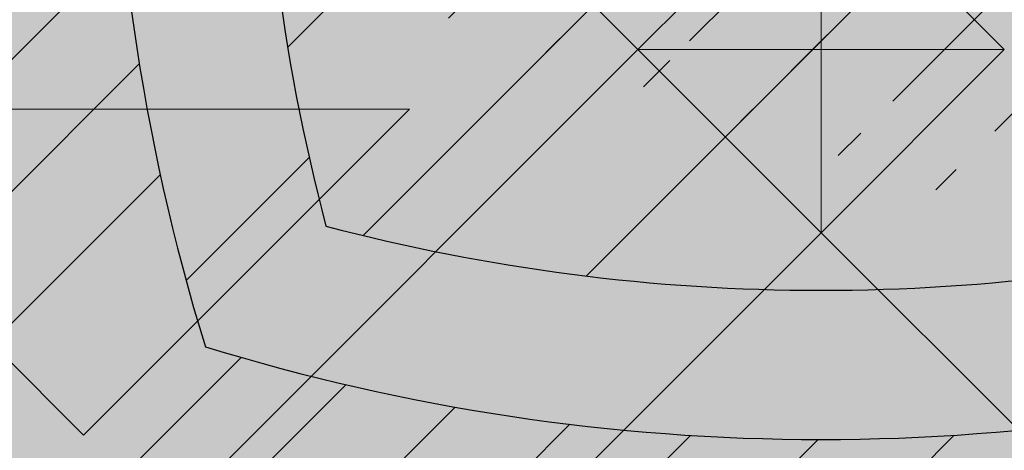
# Model space of a CAD drawing. Units: inches. Extents: x 844 to 2234, y 346 to 1084.
# Tile 10 of 93: x 1121.143 to 1123.249, y 690.263 to 691.183. Entities that reach past the tile are written whole.
import ezdxf

# ---------------------------------------------------------------- set-up
doc = ezdxf.new("R2010")
doc.units = ezdxf.units.IN
doc.header["$MEASUREMENT"] = 0
for name, color, linetype, lineweight in [('A-ANNO-DIMS', 2, 'Continuous', 18), ('furniture', 8, 'Continuous', 18), ('RA-AP-01$0$INT', 35, 'Continuous', 5)]:
    doc.layers.add(name, color=color, linetype=linetype, lineweight=lineweight)
doc.layers.add('RA-AP-01$0$FURN', color=3, linetype='Continuous')
doc.layers.add('RA-AP-01$0$WOOD', color=64, linetype='Continuous')
doc.styles.get("Standard").update_dxf_attribs({"font": 'arial.ttf'})
doc.dimstyles.get("Standard").update_dxf_attribs({"dimtxt": 6, "dimasz": 3, "dimexe": 0.18, "dimexo": 0.0625, "dimgap": 0.09, "dimtad": 0, "dimtih": 1, "dimtoh": 1, "dimdec": 1, "dimzin": 0, "dimdsep": 46, "dimlunit": 3, "dimtxsty": 'Standard', "dimblk": 'ARCHTICK', "dimcen": 0.09, "dimadec": 0, "dimazin": 0, "dimtfac": 1, "dimtdec": 1, "dimtofl": 0, "dimtmove": 0, "dimatfit": 3, "dimfxl": 1, "dimtolj": 1, "dimtzin": 0, "dimarcsym": 0})

# ---------------------------------------------------------------- blocks, each defined once
blk = doc.blocks.new('A$C18D01794')
at = {"layer": 'RA-AP-01$0$INT'}
h = blk.add_hatch(color=256, dxfattribs=at)
h.paths.add_polyline_path([(4.585917135068449, -6.356712009588271), (4.555206456959269, -6.35671200958746), (4.555206456959137, -6.387422687716308), (4.874495778835233, -6.706712009592356), (4.90520645695423, -6.676001331474049)])
h.paths.add_polyline_path([(5.255206456948813, -6.387422687716306), (5.255206456948682, -6.356712009605972), (5.224495778822613, -6.356712009605161), (4.905206456953498, -6.676001331474273), (4.935917135072151, -6.706712009592924)])
h.paths.add_polyline_path([(4.935917135072559, -6.706712009592068), (4.905206456953564, -6.737422687710376), (5.255206456951813, -7.087422687708613), (5.255206456951549, -7.026001331471008)])
h.paths.add_polyline_path([(4.555206456956399, -7.026001331471013), (4.555206456956134, -7.087422687708616), (4.905206456953821, -6.737422687710943), (4.874495778835166, -6.70671200959229)])
h = blk.add_hatch(color=256, dxfattribs=at)
h.paths.add_polyline_path([(4.585917135068448, -6.356712009588273), (4.614201406330596, -6.356712009589021), (4.668846067270487, -6.411356670531338), (4.723490728212344, -6.356712009591912), (4.771774999457151, -6.35671200959319), (4.826419660396886, -6.411356670535356), (4.862780050090322, -6.374996280843536), (4.844495778842715, -6.356712009595112), (4.862780050090411, -6.356712009595595), (4.905206456960182, -6.399138416468211), (4.947632863832445, -6.356712009597838), (4.965917135079675, -6.356712009598322), (4.947632863831759, -6.374996280845421), (4.983993253523576, -6.411356670538857), (5.038637914464627, -6.356712009600247), (5.08692218571208, -6.356712009601523), (5.141566846649976, -6.411356670541852), (5.196211507589851, -6.356712009604411), (5.224495778822615, -6.356712009605161), (4.905206456953975, -6.676001331473793)])
h.paths.add_polyline_path([(4.895206456956031, -6.637717060225675), (4.895206456958921, -6.528427738347902), (4.840561796018589, -6.583072399285802)], flags=16)
h.paths.add_polyline_path([(4.915206456955638, -6.637717060226121), (4.969851117895509, -6.583072399288678), (4.915206456957609, -6.528427738348344)], flags=16)
h.paths.add_polyline_path([(4.826419660395175, -6.568930263661755), (4.881064321335613, -6.514285602723745), (4.771774999456703, -6.514285602720857)], flags=16)
h.paths.add_polyline_path([(4.983993253519558, -6.568930263665262), (5.038637914460456, -6.514285602726792), (4.929348592581548, -6.514285602724816)], flags=16)
h.paths.add_polyline_path([(4.881064321336025, -6.494285602723742), (4.826419660397532, -6.439640941782821), (4.771774999457062, -6.494285602720859)], flags=16)
h.paths.add_polyline_path([(4.929348592582019, -6.494285602724817), (5.038637914460982, -6.494285602726792), (4.983993253522945, -6.439640941786327)], flags=16)
h.paths.add_polyline_path([(4.895206456960191, -6.480143467100443), (4.895206456962115, -6.407422687715913), (4.876922185715016, -6.389138416467584), (4.840561796021581, -6.425498806159401)], flags=16)
h.paths.add_polyline_path([(4.915206456958487, -6.480143467100889), (4.969851117899527, -6.425498806162279), (4.933490728206909, -6.389138416468043), (4.9152064569598, -6.40742268771434)], flags=16)
h.paths.add_polyline_path([(4.757632863832376, -6.480143467096812), (4.812277524772842, -6.425498806158772), (4.757632863834348, -6.370854145217844)], flags=16)
h.paths.add_polyline_path([(4.737632863832376, -6.480143467096286), (4.737632863834348, -6.370854145217375), (4.682988202893906, -6.425498806155385)], flags=16)
h.paths.add_polyline_path([(5.05278005008503, -6.480143467103376), (5.052780050087917, -6.370854145224413), (4.998135389146995, -6.425498806162908)], flags=16)
h.paths.add_polyline_path([(5.072780050085024, -6.480143467103744), (5.127424711025931, -6.42549880616527), (5.072780050087916, -6.370854145224832)], flags=16)
h.paths.add_polyline_path([(4.935917135072783, -6.706712009592292), (5.255206456948811, -6.387422687716309), (5.255206456948932, -6.415706958964177), (5.200561796010279, -6.470351619902839), (5.255206456949403, -6.524996280841948), (5.25520645694961, -6.5732805520894), (5.200561796009787, -6.627925213029239), (5.236922185702417, -6.664285602721864), (5.255206456949919, -6.646001331474357), (5.255206456949998, -6.664285602721898), (5.212780050078687, -6.706712009592262), (5.25520645695036, -6.749138416463932), (5.255206456950438, -6.767422687711313), (5.236922185702424, -6.749138416463297), (5.200561796009796, -6.785498806155928), (5.255206456950753, -6.840143467096874), (5.25520645695096, -6.888427738341682), (5.200561796010322, -6.943072399282328), (5.255206456951428, -6.997717060223427), (5.255206456951547, -7.026001331471006)])
h.paths.add_polyline_path([(5.042988202883395, -6.785498806155427), (5.097632863823085, -6.840143467095101), (5.097632863822622, -6.730854145216193)], flags=16)
h.paths.add_polyline_path([(5.028846067259663, -6.771356670531693), (5.083490728198774, -6.716712009592573), (4.974201406321001, -6.716712009593042)], flags=16)
h.paths.add_polyline_path([(5.117632863823087, -6.840143467095186), (5.172277524762331, -6.785498806155926), (5.11763286382262, -6.730854145216225)], flags=16)
h.paths.add_polyline_path([(5.08349072819877, -6.696712009593886), (5.028846067259652, -6.642067348654775), (4.974201406320998, -6.696712009593438)], flags=16)
h.paths.add_polyline_path([(5.131774999446817, -6.854285602718917), (5.186419660386065, -6.799640941779662), (5.241064321325782, -6.854285602719365)], flags=17)
h.paths.add_polyline_path([(5.131774999446228, -6.716712009592374), (5.186419660386065, -6.771356670532194), (5.222780050079488, -6.734996280838764), (5.204495778832781, -6.716712009592063)], flags=16)
h.paths.add_polyline_path([(5.097632863822613, -6.682569873970264), (5.097632863823061, -6.573280552091354), (5.042988202883383, -6.627925213031044)], flags=16)
h.paths.add_polyline_path([(5.131774999446899, -6.874285602718915), (5.241064321325809, -6.874285602719364), (5.186419660386591, -6.928930263658598)], flags=17)
h.paths.add_polyline_path([(5.131774999446226, -6.696712009594078), (5.204495778830767, -6.696712009594374), (5.22278005007868, -6.67842773834687), (5.186419660386049, -6.642067348654249)], flags=16)
h.paths.add_polyline_path([(5.11763286382262, -6.682569873970225), (5.17227752476232, -6.627925213030515), (5.117632863823064, -6.573280552091267)], flags=16)
h.paths.add_polyline_path([(5.186419660386069, -6.613783077405491), (5.241064321325754, -6.559138416465795), (5.131774999446791, -6.559138416466263)], flags=16)
h.paths.add_polyline_path([(5.131774999446872, -6.539138416466263), (5.24106432132578, -6.539138416465794), (5.186419660386554, -6.484493755526573)], flags=16)
h.paths.add_polyline_path([(5.255206456951811, -7.08742268770861), (5.255206456951895, -7.106712009588038), (4.555206456956052, -7.106712009588038), (4.555206456956136, -7.087422687708617), (4.905206456953973, -6.737422687710788)])
h.paths.add_polyline_path([(4.983993253513404, -6.8444937555241), (4.92934859257295, -6.899138416462108), (5.03863791445186, -6.899138416465014)], flags=16)
h.paths.add_polyline_path([(4.969851117889988, -6.83035161990006), (4.915206456952556, -6.775706958960171), (4.915206456949648, -6.884996280837944)], flags=16)
h.paths.add_polyline_path([(4.929348592572535, -6.919138416462105), (4.983993253511019, -6.973783077403037), (5.038637914451496, -6.919138416465012)], flags=16)
h.paths.add_polyline_path([(5.052780050074912, -6.93328055208906), (4.998135389134438, -6.987925213027088), (5.052780050072919, -7.042569873968025)], flags=16)
h.paths.add_polyline_path([(5.07278005007491, -6.933280552089588), (5.072780050072918, -7.042569873968497), (5.127424711013374, -6.987925213030498)], flags=16)
h.paths.add_polyline_path([(4.89520645695295, -6.775706958959721), (4.840561796013067, -6.830351619897157), (4.895206456950961, -6.884996280837494)], flags=16)
h.paths.add_polyline_path([(4.915206456948365, -6.933280552085403), (4.915206456946434, -7.006001331471951), (4.933490728192729, -7.024285602719066), (4.969851117886972, -6.987925213026453)], flags=16)
h.paths.add_polyline_path([(4.881064321327021, -6.899138416461022), (4.82641966038902, -6.84449375552057), (4.771774999448108, -6.899138416459029)], flags=16)
h.paths.add_polyline_path([(4.895206456950073, -6.933280552084951), (4.840561796009022, -6.987925213023558), (4.876922185700835, -7.024285602716997), (4.895206456948749, -7.006001331469487)], flags=16)
h.paths.add_polyline_path([(4.983993253510392, -7.0020673486505), (4.947632863816944, -7.038427738342319), (4.965917135064043, -7.05671200959023), (5.038637914448995, -7.056712009591555)], flags=16)
h.paths.add_polyline_path([(4.881064321326543, -6.91913841646102), (4.771774999447578, -6.919138416459031), (4.826419660385607, -6.973783077399508)], flags=16)
h.paths.add_polyline_path([(4.905206456946447, -7.014285602717636), (4.862780050074785, -7.056712009588352), (4.947632863816685, -7.056712009589775)], flags=16)
h.paths.add_polyline_path([(5.14156684663679, -7.002067348654549), (5.086922185696452, -7.056712009592438), (5.196211507574223, -7.056712009594425)], flags=16)
h.paths.add_polyline_path([(4.8264196603837, -7.002067348646972), (4.771774999442643, -7.056712009585575), (4.8444957788276, -7.056712009587508), (4.862780050075511, -7.038427738340416)], flags=16)
h.paths.add_polyline_path([(4.812277524760289, -6.98792521302292), (4.757632863822258, -6.933280552082447), (4.757632863819352, -7.042569873961408)], flags=16)
h.paths.add_polyline_path([(4.73763286382226, -6.933280552082079), (4.682988202881349, -6.987925213020536), (4.737632863819352, -7.04256987396099)], flags=16)
h.paths.add_polyline_path([(4.723490728195188, -7.056712009584289), (4.668846067257299, -7.002067348643949), (4.614201406317417, -7.056712009581383)], flags=16)
h.paths.add_polyline_path([(4.597632863829262, -6.706712009592262), (4.555206456957951, -6.664285602721896), (4.555206456958029, -6.646001331474357), (4.573490728205535, -6.664285602721864), (4.609851117898167, -6.627925213029238), (4.555206456958338, -6.573280552089402), (4.555206456958546, -6.524996280841952), (4.60985111789767, -6.470351619902839), (4.555206456959015, -6.415706958964177), (4.555206456959138, -6.387422687716309), (4.874495778835167, -6.70671200959229), (4.5552064569564, -7.026001331471015), (4.555206456956523, -6.997717060223433), (4.609851117897629, -6.94307239928233), (4.555206456956988, -6.888427738341681), (4.555206456957198, -6.840143467096881), (4.609851117898153, -6.78549880615593), (4.573490728205528, -6.749138416463297), (4.555206456957507, -6.76742268771132), (4.555206456957585, -6.749138416463933)])
h.paths.add_polyline_path([(4.712780050085332, -6.730854145216195), (4.712780050084863, -6.840143467095105), (4.767424711024555, -6.785498806155427)], flags=16)
h.paths.add_polyline_path([(4.726922185709173, -6.716712009592573), (4.781566846648288, -6.771356670531693), (4.836211507586949, -6.716712009593043)], flags=16)
h.paths.add_polyline_path([(4.692780050085327, -6.730854145216225), (4.638135389145619, -6.785498806155928), (4.692780050084865, -6.840143467095185)], flags=16)
h.paths.add_polyline_path([(4.726922185709182, -6.696712009593886), (4.836211507586949, -6.696712009593436), (4.7815668466483, -6.642067348654773)], flags=16)
h.paths.add_polyline_path([(4.678637914461726, -6.71671200959237), (4.605917135075169, -6.716712009592063), (4.587632863828464, -6.734996280838766), (4.623993253521887, -6.771356670532195)], flags=16)
h.paths.add_polyline_path([(4.712780050085336, -6.68256987397026), (4.767424711024568, -6.627925213031042), (4.71278005008489, -6.573280552091352)], flags=16)
h.paths.add_polyline_path([(4.678637914461726, -6.696712009594076), (4.623993253521899, -6.642067348654247), (4.587632863829271, -6.67842773834687), (4.605917135077185, -6.696712009594376)], flags=16)
h.paths.add_polyline_path([(4.692780050085336, -6.682569873970228), (4.692780050084889, -6.573280552091267), (4.638135389145632, -6.627925213030515)], flags=16)
h.paths.add_polyline_path([(4.623993253521885, -6.799640941779662), (4.678637914461131, -6.854285602718915), (4.56934859258217, -6.854285602719365)], flags=17)
h.paths.add_polyline_path([(4.623993253521901, -6.613783077405509), (4.678637914461158, -6.559138416466263), (4.569348592582195, -6.559138416465795)], flags=16)
h.paths.add_polyline_path([(4.678637914461051, -6.874285602718915), (4.623993253521361, -6.928930263658598), (4.569348592582143, -6.874285602719364)], flags=17)
h.paths.add_polyline_path([(4.678637914461076, -6.539138416466263), (4.623993253521399, -6.484493755526573), (4.569348592582167, -6.539138416465796)], flags=16)
h = blk.add_hatch(color=256, dxfattribs=at)
h.paths.add_polyline_path([(4.781566846647504, -6.771356670530272), (4.836211507586161, -6.716712009591613), (4.726922185708388, -6.716712009591159)])
h.paths.add_polyline_path([(4.836211507586161, -6.696712009592008), (4.781566846647504, -6.642067348653354), (4.726922185708388, -6.69671200959247)])
h.paths.add_polyline_path([(4.76742471102377, -6.627925213029623), (4.712780050084083, -6.57328055208994), (4.712780050084542, -6.68256987396885)])
h.paths.add_polyline_path([(4.692780050084544, -6.682569873968819), (4.692780050084084, -6.573280552089856), (4.638135389144834, -6.627925213029111)])
h.paths.add_polyline_path([(4.678637914460932, -6.696712009592669), (4.623993253521102, -6.642067348652844), (4.587632863827676, -6.678427738346266), (4.605917135074382, -6.696712009592973)])
h.paths.add_polyline_path([(4.573490728204743, -6.664285602721736), (4.60985111789737, -6.627925213029108), (4.555206456957541, -6.573280552089279), (4.555206456957237, -6.646001331474231)])
h.paths.add_polyline_path([(4.623993253521098, -6.613783077405377), (4.67863791446035, -6.559138416466126), (4.56934859258139, -6.559138416465669)])
h.paths.add_polyline_path([(4.678637914460275, -6.539138416466126), (4.623993253520583, -6.48449375552644), (4.56934859258136, -6.539138416465672)])
h.paths.add_polyline_path([(4.609851117896854, -6.470351619902707), (4.555206456958196, -6.415706958964051), (4.555206456957738, -6.524996280841822)])
h.paths.add_polyline_path([(4.597632863828475, -6.706712009592775), (4.555206456957283, -6.664285602721582), (4.555206456956805, -6.749138416463489)])
h.paths.add_polyline_path([(4.678637914460932, -6.716712009590963), (4.605917135076396, -6.71671200959066), (4.587632863828479, -6.734996280838164), (4.623993253521104, -6.771356670530792)])
h.paths.add_polyline_path([(4.692780050084091, -6.840143467093776), (4.692780050084548, -6.730854145214809), (4.638135389144834, -6.785498806154524)])
h.paths.add_polyline_path([(4.767424711023772, -6.785498806154004), (4.712780050084545, -6.730854145214786), (4.712780050084089, -6.840143467093692)])
h.paths.add_polyline_path([(4.67863791446036, -6.854285602718778), (4.623993253521105, -6.799640941779527), (4.569348592581399, -6.854285602719237)])
h.paths.add_polyline_path([(4.609851117897371, -6.785498806155798), (4.573490728204743, -6.74913841646317), (4.555206456957237, -6.767422687710675), (4.555206456957548, -6.840143467095629)])
h.paths.add_polyline_path([(4.623993253520596, -6.928930263658465), (4.67863791446028, -6.874285602718778), (4.569348592581367, -6.874285602719238)])
h.paths.add_polyline_path([(4.609851117896867, -6.943072399282199), (4.555206456957749, -6.888427738343082), (4.55520645695821, -6.997717060220857)])
h = blk.add_hatch(color=256, dxfattribs=at)
h.paths.add_polyline_path([(4.905206456953579, -6.70671200959253), (4.905206456953751, -6.676001331474523), (4.874495778835229, -6.706712009592358)])
h.paths.add_polyline_path([(4.935917135071924, -6.706712009592703), (4.905206456953583, -6.706712009592529), (4.90520645695341, -6.737422687710532)])
h = blk.add_hatch(color=256, dxfattribs=at)
h.paths.add_polyline_path([(4.905206456953409, -6.737422687710532), (4.90520645695358, -6.706712009592529), (4.874495778835235, -6.706712009592359)])
h.paths.add_polyline_path([(4.935917135071928, -6.706712009592703), (4.905206456953754, -6.676001331474527), (4.905206456953582, -6.706712009592529)])
for p, q in [((4.905206456953975, -6.676001331473793), (4.585917135071132, -6.356712009590955)), ((4.905206456953975, -6.676001331473793), (5.224495778822613, -6.356712009605161)), ((4.874495778835167, -6.70671200959229), (4.555206456959136, -6.387422687716307)), ((4.726922185709182, -6.696712009593882), (4.781566846648298, -6.642067348654775)), ((4.836211507586951, -6.696712009593436), (4.781566846648298, -6.642067348654775)), ((4.874495778835233, -6.706712009592356), (4.905206456953753, -6.676001331474525)), ((4.935917135071927, -6.706712009592701), (4.905206456953751, -6.676001331474525)), ((4.905206456953753, -6.676001331474525), (4.905206456953409, -6.737422687710532)), ((4.72692218570918, -6.696712009593886), (4.836211507586951, -6.696712009593436)), ((4.874495778835167, -6.70671200959229), (4.555206456956399, -7.026001331471013)), ((4.874495778835233, -6.706712009592356), (4.905206456953409, -6.737422687710532)), ((4.874495778835233, -6.706712009592358), (4.935917135071925, -6.706712009592703)), ((4.935917135071927, -6.706712009592701), (4.905206456953407, -6.737422687710532))]:
    blk.add_line(p, q, dxfattribs=at)
blk = doc.blocks.new('A$C32926AE1')
at = {"layer": 'RA-AP-01$0$FURN'}
h = blk.add_hatch(dxfattribs=at)
h.set_pattern_fill('ANSI31', color=256, scale=0.1, style=0)
h.set_pattern_definition([(45, (0, 0), (-0.0088388347648318, 0.0088388347648318), [])])
edge = h.paths.add_edge_path(flags=16)
edge.add_arc((4.904771284329206, 4.246793130718756), 0.2603971832811541, 75.22398030683196, 104.7760196931204)
edge.add_arc((4.904771284329206, 4.246793130718756), 0.2603971832811541, 75.223980306832, 104.77601969312039, ccw=False)
edge = h.paths.add_edge_path(flags=16)
edge.add_arc((4.904771284329206, 4.067062675376612), 0.2603971832811541, 255.2239803068796, 284.776019693168)
edge.add_arc((4.904771284329206, 4.067062675376612), 0.2603971832811541, 255.22398030687958, 284.77601969316805, ccw=False)
edge = h.paths.add_edge_path(flags=0)
edge.add_arc((4.904771284329206, 4.067062675376612), 0.2603971832811541, 255.2239803068796, 284.776019693168)
edge.add_arc((4.904771284329206, 4.067062675376612), 0.2603971832811541, 255.22398030687958, 284.77601969316805, ccw=False)
edge = h.paths.add_edge_path(flags=0)
edge.add_arc((4.904771284329206, 4.067062675376612), 0.2603971832811541, 255.2239803068796, 284.776019693168)
edge.add_arc((4.904771284329206, 4.067062675376612), 0.2603971832811541, 255.22398030687958, 284.77601969316805, ccw=False)
edge = h.paths.add_edge_path()
edge.add_arc((4.604388392048174, 4.588829985554312), 0.1599999999999918, 342.3781640246255, 354.4317409793762)
edge.add_arc((5.090145208887507, 4.43216705527679), 0.3503971832811637, 162.0091218307731, 180.3186872093483)
edge.add_arc((5.205154176610243, 4.588829985554953), 0.1599999999999917, 185.5682590208461, 197.6218359767349)
edge.add_arc((4.904771284329229, 4.246793130718735), 0.3503971832811761, 72.00912183053516, 107.9908781690354)
edge.add_arc((9.535952835716557, 4.28682295566602), 4.798342501046485, 178.2875002453811, 181.5576802719453)
edge.add_arc((4.719397359771122, 4.43216705527679), 0.3503971832811637, 359.6813127906516, 377.9908781692269)
edge.add_arc((9.535967292294904, 4.286822350292874), 4.778371420254705, 178.2965938931842, 181.5667745797229)
edge.add_arc((4.719397359771122, 4.43216705527679), 0.3303971832811637, 359.6813127906516, 377.9908781692269)
edge.add_arc((0.2735752763637294, 4.286822350292874), 4.7783714202547, 358.4332254202771, 361.7034061068158)
edge.add_arc((5.061434214606998, 4.732549947558029), 0.1600000000000254, 252.3781640250584, 264.4317409792362)
edge.add_arc((4.748108354051257, 4.732549947558012), 0.1600000000000541, 275.5682590208426, 287.6218359759532)
edge.add_arc((4.604388392048115, 4.588829985554317), 0.1800000000000505, 342.3567572500182, 349.3735009646207)
edge.add_arc((5.205154176610254, 4.588829985554976), 0.1800000000000069, 190.6264990356027, 197.6432427513933)
edge.add_arc((5.061434214607106, 4.732549947558013), 0.1800000000000424, 252.3567572496606, 259.3735009644582)
edge.add_arc((4.904771284329208, 4.246793130718737), 0.3303971832811676, 71.99844483668534, 108.0015551637021)
edge.add_arc((4.748108354051414, 4.732549947558045), 0.1800000000000547, 280.6264990355479, 287.6432427495938)
edge.add_arc((5.090145208887514, 4.432167055276789), 0.2803971832811691, 162.8706300666893, 180.816523289902)
edge.add_arc((4.719397359771136, 4.432167055276689), 0.2803971832811534, 359.183476710103, 377.1293699333214)
edge.add_arc((4.904771284329222, 4.246793130718737), 0.2803971832811769, 72.87063006672916, 107.1293699332334)
edge.add_arc((5.090145208887522, 4.432167055276788), 0.2603971832811776, 165.2239803068007, 180.9953123810312)
edge.add_arc((4.719397359771141, 4.432167055276699), 0.2603971832811458, 359.0046876189768, 374.7760196932087)
edge.add_arc((5.090145208887507, 4.43216705527679), 0.3303971832811637, 162.0091218307731, 180.3186872093483)
edge.add_arc((9.53595427642584, 4.285015535491528), 4.728345371032053, 178.265043920078, 181.5679956281801)
edge.add_arc((0.2735882922327999, 4.285015535491582), 4.728345371032045, 358.4320043718193, 361.7349560799204)
edge.add_arc((9.535953591267507, 4.284458026472751), 4.708343996644348, 178.2573054306777, 181.5704995759608)
edge.add_arc((0.273588977391114, 4.284458026472785), 4.708343996644358, 358.4295004240388, 361.7426945693213)
edge.add_arc((0.2735889773911131, 4.029397779622582), 4.708343996644359, 358.2573054306787, 361.5704995759613)
edge.add_arc((9.535953591267518, 4.029397779622618), 4.708343996644359, 178.4295004240391, 181.7426945693223)
edge.add_arc((0.2735882922327901, 4.028840270603786), 4.728345371032054, 358.2650439200796, 361.5679956281808)
edge.add_arc((9.53595427642584, 4.028840270603841), 4.728345371032054, 178.4320043718199, 181.7349560799219)
edge.add_arc((0.2735752763637302, 4.027033455802493), 4.778371420254699, 358.2965938931842, 361.5667745797229)
edge.add_arc((4.719397359771122, 3.881688750818578), 0.3303971832811637, 342.0091218307731, 360.3186872093484)
edge.add_arc((5.090145208887507, 3.881688750818578), 0.3303971832811637, 179.6813127906516, 197.9908781692269)
edge.add_arc((9.535967292294904, 4.027033455802493), 4.778371420254705, 178.433225420277, 181.7034061068158)
edge.add_arc((4.719397359771122, 3.881688750818578), 0.3503971832811637, 342.0091218307731, 360.3186872093484)
edge.add_arc((9.53595283571655, 4.027032850429349), 4.79834250104648, 178.4423197280546, 181.7124997546188)
edge.add_arc((4.719397359771141, 3.881688750818669), 0.2603971832811458, 345.2239803067913, 360.9953123810232)
edge.add_arc((5.090145208887522, 3.88168875081858), 0.2603971832811776, 179.0046876189687, 194.7760196931993)
edge.add_arc((4.904771284329222, 4.067062675376631), 0.2803971832811769, 252.8706300667665, 287.1293699332708)
edge.add_arc((4.719397359771136, 3.881688750818678), 0.2803971832811534, 342.8706300666787, 360.8165232898969)
edge.add_arc((5.090145208887514, 3.881688750818579), 0.2803971832811691, 179.183476710098, 197.1293699333106)
edge.add_arc((4.748108354051414, 3.581305858537323), 0.1800000000000547, 72.3567572504062, 79.37350096445199)
edge.add_arc((4.904771284329208, 4.067062675376631), 0.3303971832811676, 251.9984448362979, 288.0015551633146)
edge.add_arc((5.061434214607106, 3.581305858537355), 0.1800000000000424, 100.6264990355418, 107.6432427503394)
edge.add_arc((5.205154176610254, 3.725025820540392), 0.1800000000000069, 162.3567572486066, 169.3735009643972)
edge.add_arc((4.604388392048115, 3.725025820541051), 0.1800000000000505, 10.62649903537925, 17.64324274998182)
edge.add_arc((4.748108354051257, 3.581305858537356), 0.1600000000000541, 72.37816402404681, 84.43174097915735)
edge.add_arc((4.904771284329229, 4.067062675376632), 0.3503971832811761, 252.0091218309645, 287.9908781694648)
edge.add_arc((5.061434214606998, 3.581305858537339), 0.1600000000000254, 95.56825902076373, 107.6218359749416)
edge.add_arc((5.205154176610243, 3.725025820540414), 0.1599999999999917, 162.3781640232651, 174.4317409791539)
edge.add_arc((5.090145208887507, 3.881688750818578), 0.3503971832811637, 179.6813127906516, 197.9908781692269)
edge.add_arc((4.604388392048174, 3.725025820541056), 0.1599999999999918, 5.568259020623824, 17.62183597537444)
edge.add_arc((0.2735897329420762, 4.28682295566602), 4.798342501046482, 358.4423197280547, 361.7124997546188)
edge.add_arc((0.2735897329420691, 4.027032850429348), 4.798342501046489, 358.2875002453812, 361.5576802719453)
at = {"layer": 'RA-AP-01$0$WOOD'}
h = blk.add_hatch(color=256, dxfattribs=at)
h.dxf.hatch_style = 1
h.paths.add_polyline_path([(5.157430609644524, 4.573483066760929, -0.1009492694046607), (5.155401577623758, 4.593365984175333, -0.1842662638101597), (5.172249623284174, 4.638795604568598, 0.2056608120311276), (5.179560981299304, 4.661316324430096, 0.3614336704623542), (5.134352340494423, 4.706524965234944, 0.2056608120311297), (5.111831620632933, 4.699213607219793, -0.1842662638101113), (5.066402000239693, 4.682365561559342, -0.1055311479399994), (5.045656153913092, 4.68467289944697, 0.1567636581983829), (4.763886414745334, 4.684672899446966, -0.1055311479399895), (4.743140568418733, 4.68236556155934, -0.1842662638100833), (4.6977109480255, 4.69921360721979, 0.2056608120302612), (4.675190228164109, 4.706524965234949, 0.3614336704708441), (4.629981587358889, 4.66131632442871, 0.2056608120245944), (4.637292945374126, 4.638795604567974, -0.1842662638101024), (4.654140991034615, 4.59336598417475, -0.1009492694055169), (4.652111959013835, 4.573483066760181, 0.021410119221476), (4.629748025606143, 4.156712009541676, 0.0214101192214795), (4.652111959013809, 3.739940952323101, -0.1009492694059586), (4.654140991034615, 3.720058034908448, -0.1842662638100975), (4.637292945374126, 3.674628414515226, 0.2056608120245705), (4.629981587358889, 3.652107694654492, 0.3614336704708879), (4.675190228164113, 3.606899053848249, 0.2056608120302384), (4.697710948025501, 3.614210411863408, -0.1842662638100995), (4.743140568418738, 3.63105845752386, -0.1055311479402541), (4.763886414745388, 3.628751119636215, 0.1567636581983776), (5.045656153913137, 3.628751119636244, -0.1055311479397538), (5.066402000239692, 3.631058457523857, -0.1842662638101067), (5.111831620632931, 3.614210411863407, 0.2056608120310924), (5.134352340494417, 3.606899053848256, 0.3614336704624001), (5.179560981299307, 3.652107694653103, 0.2056608120311314), (5.172249623284175, 3.6746284145146, -0.1842662638101402), (5.155401577623758, 3.72005803490786, -0.1009492694051366), (5.15743060964455, 3.739940952322354, 0.0214101192215073), (5.179794543052287, 4.156712009541468, 0.0214101192215252)])
h.paths.add_polyline_path([(4.639748609479751, 4.156712009541513, 0.0213537860821624), (4.661970494867118, 3.741887061152232, -0.094075836301374), (4.664143710413708, 3.7196126951003, -0.1824818158568985), (4.644813765429836, 3.668037719127816, 0.2056608120245319), (4.639939526753007, 3.653023905887301, 0.3614336704710246), (4.676106439397173, 3.616856993242342, 0.2056608120302234), (4.691120252638095, 3.621731231919122, -0.1824818158602558), (4.742695228611606, 3.641061176902986, -0.1029891339458722), (4.766991894714349, 3.638256818950944, 0.156709409989566), (5.042550673941472, 3.638256818950105, -0.102989133958497), (5.066847340047078, 3.641061176902949, -0.1824818158594995), (5.118422316020358, 3.621731231919103, 0.2056608120311416), (5.133436129261316, 3.616856993242346, 0.3614336704621468), (5.169603041905217, 3.653023905886178, 0.2056608120310986), (5.164728803228477, 3.668037719127177, -0.1824818158565612), (5.145398858244737, 3.719612695099578, -0.0940758363009313), (5.147572073791232, 3.741887061151398, 0.0213537860822023), (5.169793959178681, 4.156712009541451, 0.0213537860822226), (5.147572073791203, 4.571536957931898, -0.0940758363005034), (5.145398858244737, 4.59381132398362, -0.1824818158565587), (5.164728803228476, 4.645386299956021, 0.2056608120311045), (5.169603041905216, 4.66040011319702, 0.3614336704621845), (5.133436129261313, 4.696567025840856, 0.2056608120310773), (5.118422316020359, 4.691692787164098, -0.182481815859508), (5.066847340047078, 4.67236284218025, -0.1029891339584606), (5.04255067394148, 4.675167200133092, 0.156709409989566), (4.766991894714357, 4.675167200132257, -0.1029891339458842), (4.742695228611611, 4.672362842180213, -0.1824818158602725), (4.691120252638095, 4.691692787164077, 0.2056608120302152), (4.676106439397174, 4.696567025840858, 0.3614336704710363), (4.639939526753005, 4.660400113195899, 0.2056608120245495), (4.644813765429837, 4.645386299955384, -0.1824818158568934), (4.664143710413708, 4.593811323982902, -0.0940758363009187), (4.661970494867149, 4.571536957931074, 0.021353786082177)], flags=16)
h.paths.add_polyline_path([(5.129794543052235, 4.432167055276933, -0.0141661062790638), (5.130152669293814, 4.156927903047693, -0.0141661062790647), (5.129794543052234, 3.881688750818433, -0.0785247771143638), (5.10979738006795, 3.755143611847103, 0.0945969212073497), (5.105408519571111, 3.717898134952927, 0.1043170707844957), (5.116074640131521, 3.670385395016088, 0.1043170707864965), (5.068561900193738, 3.681051515576561, 0.09459692119553), (5.031316423304057, 3.676662655080835, -0.1580239521427272), (4.778226145355827, 3.676662655080367, 0.0945969211986668), (4.740980668464973, 3.681051515576592, 0.1043170707882822), (4.693467928526415, 3.670385395015844, 0.1043170707867916), (4.704134049087309, 3.717898134953662, 0.0945969211972894), (4.69974518859162, 3.755143611844042, -0.0785247771163196), (4.679748025606343, 3.881688750818406, -0.0141661062790663), (4.679389899364763, 4.156927903047693, -0.0141661062790672), (4.679748025606343, 4.432167055276998, -0.0785247771163064), (4.699745188591625, 4.55871219425134, 0.094596921197333), (4.704134049087308, 4.595957671141738, 0.1043170707867205), (4.693467928526416, 4.643470411079523, 0.1043170707882628), (4.740980668464965, 4.632804290518776, 0.0945969211988114), (4.778226145355874, 4.637193151015016, -0.158023952142669), (5.031316423304015, 4.637193151014546, 0.0945969211956361), (5.068561900193736, 4.632804290518806, 0.1043170707864979), (5.11607464013152, 4.643470411079278, 0.1043170707844617), (5.105408519571112, 4.595957671142455, 0.0945969212074597), (5.109797380067959, 4.558712194248236, -0.0785247771143467)], flags=0)
h.paths.add_polyline_path([(5.119794532311105, 4.432259799204851, -0.0142000800617244), (5.120156169157484, 4.156927903047701, -0.0142000800617277), (5.119794532311105, 3.881596006890482, -0.0784894509520253), (5.100273383573699, 3.758192358677797, 0.0940138827242913), (5.095413455884425, 3.717477693979438, 0.0606271852308753), (5.099615656341024, 3.686844378806616, 0.0606271852322524), (5.068982341167493, 3.691046579263239, 0.0940138827010453), (5.028267676478798, 3.686186651576848, -0.1580706864508061), (4.781274892180912, 3.686186651576435, 0.0940138827026903), (4.740560227491556, 3.691046579263279, 0.0606271852339895), (4.709926912317155, 3.686844378806508, 0.0606271852329405), (4.714129112773991, 3.717477693980356, 0.094013882701304), (4.709269185087677, 3.758192358669163, -0.0784894509577193), (4.689748036347473, 3.881596006890469, -0.014200080061729), (4.689386399501094, 4.156927903047709, -0.0142000800617217), (4.689748036347473, 4.432259799204808, -0.078489450957724), (4.709269185087651, 4.555663447426125, 0.0940138827014585), (4.714129112773992, 4.596378112114996, 0.0606271852329731), (4.709926912317154, 4.62701142728886, 0.0606271852340196), (4.74056022749157, 4.622809226832087, 0.0940138827024997), (4.781274892180847, 4.627669154518912, -0.1580706864508359), (5.028267676478777, 4.627669154518526, 0.0940138827010946), (5.068982341167492, 4.622809226832129, 0.060627185232254), (5.099615656341024, 4.627011427288751, 0.0606271852308727), (5.095413455884425, 4.59637811211593, 0.0940138827241088), (5.100273383573675, 4.555663447417647, -0.0784894509520978)], flags=0)
h.paths.add_polyline_path([(5.06978912287499, 4.430218106756144, -0.014241683694547), (5.070173729147532, 4.156927903047672, -0.0142416836945458), (5.06978912287499, 3.883637699339223, -0.0800609523125196), (5.052662118612511, 3.773463122773442, 0.0526421978001116), (5.04590916754064, 3.740550867606997, 0.0526421977992423), (5.012996912374707, 3.73379791653534, -0.1583028414718258), (4.796545656286308, 3.73379791653451, 0.0526421978034211), (4.763633401117837, 3.740550867607021, 0.0526421978018622), (4.756880450045755, 3.773463122774558, -0.0800609523117106), (4.739753445783639, 3.883637699339268, -0.0142416836945435), (4.739368839511098, 4.156927903047671, -0.0142416836945477), (4.739753445783639, 4.430218106756155, -0.0800609523116345), (4.75688045004574, 4.540392683320762, 0.052642197801941), (4.763633401117837, 4.573304938488346, 0.0526421978035071), (4.796545656286361, 4.580057889560873, -0.1583028414717561), (5.012996912374669, 4.580057889560039, 0.0526421977993048), (5.04590916754064, 4.57330493848837, 0.0526421978002057), (5.052662118612529, 4.540392683321868, -0.080060952312477)], flags=0)
h.paths.add_polyline_path([(5.049789715110557, 4.43038092723357, -0.0143097550741839), (5.05018085590259, 4.156927903047715, -0.0143097550741854), (5.049789715110558, 3.883474878861827, -0.0800685599149176), (5.03362098255317, 3.779581877367999, 0.0306258898956367), (5.028241146483733, 3.758218888663947, 0.0306258898977031), (5.006878157778253, 3.75283905259408, -0.1583983521624096), (4.802664410878162, 3.752839052594731, 0.0306258898946014), (4.781301422174808, 3.758218888663924, 0.0306258898967912), (4.775921586105202, 3.779581877368794, -0.080068559914251), (4.759752853548071, 3.883474878861786, -0.0143097550741854), (4.759361712756037, 4.156927903047671, -0.0143097550741854), (4.759752853548071, 4.430380927233557, -0.0800685599142479), (4.775921586105193, 4.534273928726546, 0.0306258898968306), (4.781301422174808, 4.555636917431444, 0.0306258898945754), (4.802664410878143, 4.561016753500631, -0.1583983521624168), (5.006878157778244, 4.561016753501291, 0.0306258898977177), (5.028241146483733, 4.555636917431421, 0.0306258898958182), (5.03362098255321, 4.534273928727244, -0.080068559914796)], flags=0)
h.paths.add_polyline_path([(4.999766070382627, 4.428171244713864, -0.0143443147609634), (5.000198441819402, 4.156927903047689, -0.0143443147609612), (4.999766070382627, 3.885684561381556, -0.0784641635803329), (4.987356730658798, 3.799103304488872, -0.1506053783831347), (4.822185837999821, 3.79910330448882, -0.0784641635803318), (4.809776498276007, 3.885684561381509, -0.014344314760963), (4.809344126839227, 4.156927903047677, -0.0143443147609645), (4.809776498276007, 4.428171244713873, -0.0784641635803192), (4.822185837999822, 4.514752501606549, -0.1506053783831338), (4.987356730658798, 4.514752501606494, -0.078464163580285)], flags=0)
h.paths.add_polyline_path([(4.979755254238824, 4.42764379880488, -0.0143772539198268), (4.980205517789977, 4.156927903047693, -0.0143772539198275), (4.979755254238824, 3.886212007290489, -0.0689242507424422), (4.971183264704897, 3.815276770442801, -0.1296645318904179), (4.838359303953726, 3.815276770442746, -0.0689242507424186), (4.829787314419809, 3.886212007290419, -0.0143772539198292), (4.829337050868653, 4.156927903047653, -0.0143772539198325), (4.829787314419809, 4.427643798804946, -0.0689242507424211), (4.838359303953725, 4.498579035652621, -0.1296645318904187), (4.971183264704897, 4.498579035652565, -0.0689242507424401)], flags=0)
h = blk.add_hatch(color=256, dxfattribs=at)
h.dxf.hatch_style = 1
h.paths.add_polyline_path([(5.145398858244737, 4.59381132398362, -0.1824818158565616), (5.164728803228476, 4.645386299956021, 0.2056608120311045), (5.169603041905216, 4.66040011319702, 0.3614336704621845), (5.133436129261313, 4.696567025840856, 0.2056608120310773), (5.118422316020359, 4.691692787164098, -0.182481815859508), (5.066847340047078, 4.67236284218025, -0.1029891339584606), (5.04255067394148, 4.675167200133092, 0.156709409989566), (4.766991894714357, 4.675167200132257, -0.1029891339458842), (4.742695228611611, 4.672362842180213, -0.1824818158602725), (4.691120252638095, 4.691692787164077, 0.2056608120302152), (4.676106439397174, 4.696567025840858, 0.3614336704710363), (4.639939526753005, 4.660400113195899, 0.2056608120245495), (4.644813765429837, 4.645386299955384, -0.1824818158568934), (4.664143710413708, 4.593811323982902, -0.0940758363009187), (4.661970494867149, 4.571536957931074, 0.0213537860821772), (4.639748609479751, 4.156712009541507, 0.0213537860821625), (4.661970494867119, 3.741887061152226, -0.0940758363013071), (4.664143710413708, 3.719612695100309, -0.1824818158569294), (4.644813765429836, 3.668037719127816, 0.2056608120245319), (4.639939526753007, 3.653023905887301, 0.3614336704710246), (4.676106439397173, 3.616856993242342, 0.2056608120302234), (4.691120252638095, 3.621731231919122, -0.1824818158602558), (4.742695228611606, 3.641061176902986, -0.1029891339458722), (4.766991894714349, 3.638256818950944, 0.156709409989566), (5.042550673941472, 3.638256818950105, -0.102989133958497), (5.066847340047078, 3.641061176902949, -0.1824818158594995), (5.118422316020358, 3.621731231919103, 0.2056608120311416), (5.133436129261316, 3.616856993242346, 0.3614336704621468), (5.169603041905217, 3.653023905886178, 0.2056608120310986), (5.164728803228477, 3.668037719127177, -0.1824818158565612), (5.145398858244737, 3.719612695099578, -0.0940758363009313), (5.147572073791232, 3.741887061151398, 0.0213537860822023), (5.169793959178681, 4.156712009541451, 0.0213537860822226), (5.147572073791203, 4.571536957931898, -0.0940758363004996)])
h.paths.add_polyline_path([(5.109797380067958, 4.55871219424824, -0.0785247771143472), (5.129794543052234, 4.432167055276936, -0.0141661062790644), (5.130152669293814, 4.156927903047685, -0.014166106279066), (5.129794543052234, 3.881688750818401, -0.0785247771143517), (5.109797380067946, 3.755143611847092, 0.0945969212073132), (5.105408519571111, 3.717898134952929, 0.1043170707844995), (5.116074640131521, 3.670385395016088, 0.1043170707864965), (5.068561900193738, 3.681051515576561, 0.09459692119553), (5.031316423304057, 3.676662655080835, -0.1580239521427272), (4.778226145355827, 3.676662655080367, 0.0945969211986668), (4.740980668464973, 3.681051515576592, 0.1043170707882822), (4.693467928526415, 3.670385395015844, 0.1043170707867916), (4.704134049087309, 3.717898134953662, 0.0945969211972894), (4.69974518859162, 3.755143611844042, -0.0785247771163196), (4.679748025606343, 3.881688750818406, -0.0141661062790663), (4.679389899364763, 4.156927903047693, -0.0141661062790672), (4.679748025606343, 4.432167055276998, -0.0785247771163064), (4.699745188591625, 4.55871219425134, 0.094596921197333), (4.704134049087308, 4.595957671141738, 0.1043170707867205), (4.693467928526416, 4.643470411079523, 0.1043170707882628), (4.740980668464965, 4.632804290518776, 0.0945969211988114), (4.778226145355874, 4.637193151015016, -0.158023952142669), (5.031316423304015, 4.637193151014546, 0.0945969211956361), (5.068561900193736, 4.632804290518806, 0.1043170707864979), (5.11607464013152, 4.643470411079278, 0.1043170707844617), (5.105408519571112, 4.595957671142455, 0.0945969212074504)], flags=16)
h.paths.add_polyline_path([(5.100273383573655, 4.55566344741771, -0.0784894509521388), (5.119794532311105, 4.432259799204852, -0.0142000800617252), (5.120156169157484, 4.156927903047686, -0.014200080061726), (5.119794532311105, 3.881596006890502, -0.0784894509520446), (5.100273383573696, 3.758192358677786, 0.0940138827242721), (5.095413455884425, 3.717477693979436, 0.0606271852308692), (5.099615656341024, 3.686844378806616, 0.0606271852322522), (5.068982341167493, 3.691046579263239, 0.0940138827010453), (5.028267676478798, 3.686186651576848, -0.1580706864508061), (4.781274892180912, 3.686186651576435, 0.0940138827026903), (4.740560227491556, 3.691046579263279, 0.0606271852339895), (4.709926912317155, 3.686844378806508, 0.0606271852329405), (4.714129112773991, 3.717477693980356, 0.094013882701304), (4.709269185087677, 3.758192358669163, -0.0784894509577193), (4.689748036347473, 3.881596006890469, -0.014200080061729), (4.689386399501094, 4.156927903047709, -0.0142000800617217), (4.689748036347473, 4.432259799204808, -0.078489450957724), (4.709269185087651, 4.555663447426125, 0.0940138827014585), (4.714129112773992, 4.596378112114996, 0.0606271852329731), (4.709926912317154, 4.62701142728886, 0.0606271852340196), (4.74056022749157, 4.622809226832087, 0.0940138827024997), (4.781274892180847, 4.627669154518912, -0.1580706864508359), (5.028267676478777, 4.627669154518526, 0.0940138827010946), (5.068982341167492, 4.622809226832129, 0.060627185232254), (5.099615656341024, 4.627011427288751, 0.0606271852308727), (5.095413455884425, 4.59637811211593, 0.094013882723957)], flags=0)
h.paths.add_polyline_path([(5.04590916754064, 4.57330493848837, 0.0526421978002057), (5.052662118612529, 4.540392683321868, -0.0800609523124783), (5.06978912287499, 4.430218106756142, -0.0142416836945469), (5.070173729147532, 4.156927903047672, -0.0142416836945458), (5.06978912287499, 3.883637699339223, -0.0800609523125196), (5.052662118612511, 3.773463122773442, 0.0526421978001116), (5.04590916754064, 3.740550867606997, 0.0526421977992423), (5.012996912374707, 3.73379791653534, -0.1583028414718258), (4.796545656286308, 3.73379791653451, 0.0526421978034211), (4.763633401117837, 3.740550867607021, 0.0526421978018622), (4.756880450045755, 3.773463122774558, -0.0800609523117106), (4.739753445783639, 3.883637699339268, -0.0142416836945435), (4.739368839511098, 4.156927903047671, -0.0142416836945477), (4.739753445783639, 4.430218106756155, -0.0800609523116345), (4.75688045004574, 4.540392683320762, 0.052642197801941), (4.763633401117837, 4.573304938488346, 0.0526421978035071), (4.796545656286361, 4.580057889560873, -0.1583028414717561), (5.012996912374669, 4.580057889560039, 0.0526421977993048)], flags=0)
h.paths.add_polyline_path([(5.028241146483733, 4.555636917431422, 0.0306258898956949), (5.033620982553182, 4.534273928727329, -0.0800685599148649), (5.049789715110557, 4.430380927233569, -0.0143097550741839), (5.05018085590259, 4.156927903047715, -0.0143097550741854), (5.049789715110558, 3.883474878861827, -0.0800685599149176), (5.03362098255317, 3.779581877367999, 0.0306258898956367), (5.028241146483733, 3.758218888663947, 0.0306258898977031), (5.006878157778253, 3.75283905259408, -0.1583983521624096), (4.802664410878162, 3.752839052594731, 0.0306258898946014), (4.781301422174808, 3.758218888663924, 0.0306258898967912), (4.775921586105202, 3.779581877368794, -0.080068559914251), (4.759752853548071, 3.883474878861786, -0.0143097550741854), (4.759361712756037, 4.156927903047671, -0.0143097550741854), (4.759752853548071, 4.430380927233557, -0.0800685599142479), (4.775921586105193, 4.534273928726546, 0.0306258898968306), (4.781301422174808, 4.555636917431444, 0.0306258898945754), (4.802664410878143, 4.561016753500631, -0.1583983521624168), (5.006878157778244, 4.561016753501291, 0.0306258898977174)], flags=0)
h.paths.add_polyline_path([(4.987356730658798, 4.514752501606494, -0.0784641635803018), (4.999766070382627, 4.428171244713845, -0.0143443147609637), (5.000198441819402, 4.156927903047665, -0.0143443147609622), (4.999766070382628, 3.885684561381514, -0.0784641635802952), (4.987356730658797, 3.799103304488872, -0.1506053783831338), (4.822185837999821, 3.799103304488819, -0.0784641635803342), (4.809776498276007, 3.885684561381512, -0.0143443147609628), (4.809344126839227, 4.156927903047676, -0.0143443147609646), (4.809776498276007, 4.428171244713873, -0.0784641635803192), (4.822185837999822, 4.514752501606549, -0.1506053783831338)], flags=0)
h.paths.add_polyline_path([(4.971183264704897, 4.498579035652566, -0.0689242507424384), (4.979755254238824, 4.427643798804883, -0.0143772539198276), (4.980205517789977, 4.15692790304768, -0.0143772539198258), (4.979755254238823, 3.88621200729051, -0.0689242507424628), (4.971183264704897, 3.815276770442801, -0.129664531890417), (4.838359303953726, 3.815276770442746, -0.0689242507424186), (4.829787314419809, 3.886212007290419, -0.0143772539198292), (4.829337050868653, 4.156927903047653, -0.0143772539198325), (4.829787314419809, 4.427643798804946, -0.0689242507424211), (4.838359303953725, 4.498579035652621, -0.1296645318904187)], flags=0)
h = blk.add_hatch(dxfattribs=at)
h.set_pattern_fill('ANSI31', color=256, scale=0.05, style=0)
h.set_pattern_definition([(45, (0, 0), (-0.0044194173824159, 0.0044194173824159), [])])
h.paths.add_polyline_path([(5.130152669293814, 4.156927903047704, 0.0141661062790657), (5.129794543052234, 4.432167055276982, 0.0777827904001433), (5.110168979996553, 4.557559993161921, -0.0976515123401879), (5.105408519571111, 4.595957671142454, -0.1043170707844687), (5.116074640131522, 4.64347041107928), (5.099615656341024, 4.627011427288751, 0.0606271852308727), (5.095413455884425, 4.59637811211593, 0.0940138827241088), (5.100273383573675, 4.555663447417647, -0.0784894509520972), (5.119794532311105, 4.432259799204852, -0.0142000800617252), (5.120156169157484, 4.156927903047686, -0.014200080061726), (5.119794532311105, 3.881596006890502, -0.0784894509520446), (5.100273383573696, 3.758192358677786, 0.0940138827242721), (5.095413455884425, 3.717477693979436, 0.0606271852308692), (5.099615656341024, 3.686844378806616), (5.116074640131519, 3.67038539501609, -0.1043170707844594), (5.105408519571112, 3.717898134952912, -0.0976515123401594), (5.11016897999655, 3.756295812933435, 0.0777827904001654), (5.129794543052234, 3.881688750818409, 0.0141661062790665)])
h.paths.add_polyline_path([(5.030164222210597, 3.676291055149937, -0.0976515123472002), (5.068561900193739, 3.681051515576561, -0.1043170707864927), (5.116074640131521, 3.670385395016088), (5.099615656341024, 3.686844378806616, 0.0606271852322522), (5.068982341167493, 3.691046579263239, 0.0940138827010453), (5.028267676478798, 3.686186651576848, -0.1580706864508061), (4.781274892180912, 3.686186651576435, 0.0940138827026903), (4.740560227491556, 3.691046579263279, 0.0606271852339913), (4.709926912317154, 3.686844378806508), (4.693467928526416, 3.670385395015845, -0.1043170707882796), (4.740980668464973, 3.681051515576592, -0.0976515123427246), (4.779378346446416, 3.676291055150394, 0.156512506893803)])
h.paths.add_polyline_path([(4.689748036347473, 3.881596006890472, -0.014200080061729), (4.689386399501094, 4.156927903047712, -0.0142000800617195), (4.689748036347473, 4.432259799204768, -0.078489450957742), (4.709269185087648, 4.555663447426114, 0.0940138827014821), (4.714129112773992, 4.596378112114995, 0.0606271852329748), (4.709926912317154, 4.62701142728886), (4.693467928526414, 4.643470411079524, -0.1043170707867939), (4.704134049087309, 4.595957671141706, -0.09765151234893), (4.699373588660725, 4.557559993157876, 0.0777827903975372), (4.679748025606343, 4.432167055276987, 0.0141661062790675), (4.679389899364763, 4.156927903047675, 0.0141661062790641), (4.679748025606343, 3.88168875081843, 0.0777827903975637), (4.699373588660724, 3.756295812937497, -0.0976515123490278), (4.704134049087308, 3.717898134953629, -0.1043170707867196), (4.693467928526416, 3.670385395015845), (4.709926912317155, 3.686844378806508, 0.0606271852329413), (4.714129112773991, 3.717477693980357, 0.0940138827013084), (4.709269185087676, 3.758192358669166, -0.0784894509577192)])
h.paths.add_polyline_path([(4.779378346446434, 4.63756475094498, -0.0976515123427943), (4.740980668464964, 4.632804290518776, -0.1043170707882609), (4.693467928526416, 4.643470411079523), (4.709926912317154, 4.62701142728886, 0.0606271852340196), (4.74056022749157, 4.622809226832087, 0.0940138827024997), (4.781274892180847, 4.627669154518912, -0.1580706864508359), (5.028267676478777, 4.627669154518526, 0.0940138827010946), (5.068982341167492, 4.622809226832129, 0.060627185232254), (5.099615656341024, 4.627011427288751), (5.116074640131521, 4.643470411079279, -0.1043170707865022), (5.068561900193735, 4.632804290518806, -0.0976515123475899), (5.030164222210446, 4.637564750945479, 0.1565125068936924)])
h = blk.add_hatch(dxfattribs=at)
h.set_pattern_fill('ANSI32', color=256, scale=0.2, style=0)
h.set_pattern_definition([(45, (0, 0), (-0.0530330085889911, 0.0530330085889911), []), (45, (0.035355339, 0), (-0.0530330085889911, 0.0530330085889911), [])])
h.paths.add_polyline_path([(5.119794532311105, 4.432259799204823, 0.0777015974868765), (5.10065834347252, 4.554469821747928, -0.0968902511992216), (5.095413455884425, 4.596378112115931, -0.060627185230871), (5.099615656341024, 4.627011427288751, -0.060627185232254), (5.068982341167492, 4.622809226832129, -0.0968902512198245), (5.027074050790956, 4.628054114423209, 0.1564657949319105), (4.782468517866163, 4.628054114422785, -0.0968902512152247), (4.740560227491555, 4.622809226832088, -0.0606271852339878), (4.709926912317155, 4.627011427288859, -0.0606271852329413), (4.714129112773991, 4.596378112115011, -0.0968902512205338), (4.708884225182929, 4.554469821738175, 0.0777015974804443), (4.689748036347473, 4.43225979920482, 0.0142000800617215), (4.689386399501094, 4.156927903047726, 0.0142000800617273), (4.689748036347473, 3.88159600689052, 0.077701597480541), (4.708884225182985, 3.759385984357019, -0.096890251220082), (4.714129112773992, 3.717477693980371, -0.0606271852329731), (4.709926912317154, 3.686844378806507, -0.060627185233988), (4.740560227491554, 3.691046579263279, -0.0968902512152569), (4.782468517866175, 3.685801691672578, 0.1564657949319236), (5.027074050790988, 3.685801691672169, -0.0968902512197451), (5.068982341167491, 3.691046579263239, -0.0606271852322557), (5.099615656341024, 3.686844378806616, -0.0606271852308727), (5.095413455884425, 3.717477693979438, -0.0968902511991229), (5.100658343472507, 3.7593859843474, 0.0777015974868745), (5.119794532311105, 3.8815960068905, 0.014200080061726), (5.120156169157484, 4.156927903047685, 0.0142000800617238)])
h.paths.add_polyline_path([(5.070173729147531, 4.156927903047684, -0.0142416836945481), (5.06978912287499, 3.883637699339191, -0.0800609523125107), (5.052662118612505, 3.773463122773424, 0.0526421978000811), (5.04590916754064, 3.740550867606997, 0.0526421977993214), (5.012996912374658, 3.733797916535325, -0.1583028414717916), (4.796545656286304, 3.733797916534512, 0.0526421978034138), (4.763633401117837, 3.740550867607021, 0.0526421978018622), (4.756880450045755, 3.773463122774558, -0.0800609523117106), (4.739753445783639, 3.883637699339268, -0.0142416836945435), (4.739368839511098, 4.156927903047671, -0.0142416836945477), (4.739753445783639, 4.430218106756155, -0.0800609523116345), (4.75688045004574, 4.540392683320762, 0.052642197801941), (4.763633401117837, 4.573304938488346, 0.0526421978035071), (4.796545656286361, 4.580057889560873, -0.1583028414717561), (5.012996912374669, 4.580057889560039, 0.0526421977993048), (5.04590916754064, 4.57330493848837, 0.0526421978002057), (5.052662118612529, 4.540392683321868, -0.0800609523124783), (5.06978912287499, 4.430218106756142, -0.0142416836945463)], flags=16)
h.paths.add_polyline_path([(5.050180855902591, 4.156927903047686, -0.0143097550741856), (5.049789715110558, 3.883474878861795, -0.0800685599148126), (5.033620982553202, 3.7795818773681, 0.0306258898957837), (5.028241146483733, 3.758218888663947, 0.0306258898977031), (5.006878157778253, 3.75283905259408, -0.1583983521624096), (4.802664410878162, 3.752839052594731, 0.0306258898946014), (4.781301422174808, 3.758218888663924, 0.0306258898967912), (4.775921586105202, 3.779581877368794, -0.080068559914251), (4.759752853548071, 3.883474878861786, -0.0143097550741854), (4.759361712756037, 4.156927903047671, -0.0143097550741854), (4.759752853548071, 4.430380927233557, -0.0800685599142479), (4.775921586105193, 4.534273928726546, 0.0306258898968306), (4.781301422174808, 4.555636917431444, 0.0306258898945754), (4.802664410878143, 4.561016753500631, -0.1583983521624168), (5.006878157778244, 4.561016753501291, 0.0306258898977177), (5.028241146483733, 4.555636917431421, 0.0306258898958182), (5.03362098255321, 4.534273928727244, -0.0800685599147973), (5.049789715110557, 4.430380927233568, -0.0143097550741854)], flags=0)
h.paths.add_polyline_path([(5.000198441819402, 4.15692790304769, -0.0143443147609622), (4.999766070382627, 3.885684561381539, -0.0784641635803169), (4.987356730658798, 3.799103304488873, -0.1506053783831347), (4.822185837999821, 3.79910330448882, -0.0784641635803318), (4.809776498276007, 3.885684561381509, -0.014344314760963), (4.809344126839227, 4.156927903047677, -0.0143443147609645), (4.809776498276007, 4.428171244713873, -0.0784641635803192), (4.822185837999822, 4.514752501606549, -0.1506053783831338), (4.987356730658798, 4.514752501606494, -0.0784641635803018), (4.999766070382627, 4.428171244713845, -0.0143443147609624)], flags=0)
h.paths.add_polyline_path([(4.980205517789976, 4.156927903047707, -0.0143772539198295), (4.979755254238824, 3.886212007290466, -0.06892425074242), (4.971183264704897, 3.815276770442801, -0.129664531890417), (4.838359303953726, 3.815276770442746, -0.0689242507424186), (4.829787314419809, 3.886212007290419, -0.0143772539198292), (4.829337050868653, 4.156927903047653, -0.0143772539198325), (4.829787314419809, 4.427643798804946, -0.0689242507424211), (4.838359303953725, 4.498579035652621, -0.1296645318904187), (4.971183264704897, 4.498579035652565, -0.0689242507424418), (4.979755254238824, 4.427643798804878, -0.0143772539198259)], flags=0)
for centre, radius, start, end in [((5.090145208887514, 3.881688750818579), 0.2803971832811691, 179.183476710098, 197.1293699333106), ((5.090145208887522, 3.88168875081858), 0.2603971832811776, 179.0046876189687, 194.7760196931993), ((4.904771284329206, 4.067062675376612), 0.2603971832811541, 255.2239803068796, 284.776019693168), ((4.904771284329206, 4.067062675376612), 0.2603971832811541, 255.2239803068796, 284.776019693168), ((4.904771284329222, 4.067062675376631), 0.2803971832811769, 252.8706300667665, 287.1293699332708)]:
    blk.add_arc(centre, radius, start, end, dxfattribs=at)
blk = doc.blocks.new('A$C5D2F253E')
at = {"layer": 'RA-AP-01$0$FURN', "xscale": -0.7999999999883585, "yscale": 0.7999999999883585, "zscale": 0.8, "rotation": 90}
blk.add_blockref('A$C18D01794', (-5.687757199772477, 4.75791982714071), dxfattribs=at)
at = {"layer": 'RA-AP-01$0$WOOD', "rotation": 270}
blk.add_blockref('A$C32926AE1', (-4.161339601644158, 5.73852594588169), dxfattribs=at)
blk = doc.blocks.new('_ArchTick')
at = {"color": 0, "linetype": 'ByBlock', "const_width": 0.15}
blk.add_lwpolyline([(-0.5, -0.5), (0.5, 0.5)], dxfattribs=at)
blk = doc.blocks.new('*D144')
at = {"layer": 'A-ANNO-DIMS', "color": 0, "lineweight": -2, "transparency": 16777216}
for p, q in [((1096.615948, 439.3732739999999), (1096.615948, 1074.743301)), ((1143.115948, 492.373274), (1143.115948, 1074.743301)), ((1096.615948, 1074.563301), (1102.481950728513, 1074.563301)), ((1143.115948, 1074.563301), (1137.249945271487, 1074.563301))]:
    blk.add_line(p, q, dxfattribs=at)
at = {"layer": 'Defpoints', "color": 0, "transparency": 16777216}
for p in [(1143.115948, 1074.563301), (1143.115948, 492.3107739999999), (1096.615948, 439.3107739999999)]:
    blk.add_point(p, dxfattribs=at)
at = {"layer": 'A-ANNO-DIMS', "color": 0, "lineweight": -2, "transparency": 16777216, "xscale": 3, "yscale": 3, "zscale": 3, "rotation": 180}
blk.add_blockref('_ArchTick', (1096.615948, 1074.563301), dxfattribs=at)
at = {"layer": 'A-ANNO-DIMS', "color": 0, "lineweight": -2, "transparency": 16777216, "xscale": 3, "yscale": 3, "zscale": 3}
blk.add_blockref('_ArchTick', (1143.115948, 1074.563301), dxfattribs=at)
at = {"layer": 'A-ANNO-DIMS', "color": 0, "transparency": 16777216, "insert": (1119.865948, 1074.563301), "char_height": 6, "attachment_point": 5}
blk.add_mtext('\\A1;3\'-10 1/2"', dxfattribs=at)

msp = doc.modelspace()

# ---------------------------------------------------------------- block references
at = {"layer": 'furniture', "xscale": 15.94108302203742, "yscale": 15.94108302203742, "zscale": 15.94108302203742, "rotation": 90}
msp.add_blockref('A$C5D2F253E', (1136.147844094663, 696.2584716700112), dxfattribs=at)

# ---------------------------------------------------------------- dimensions: what is measured, and where the dimension line sits
at = {"layer": 'A-ANNO-DIMS'}
dim = msp.add_linear_dim(base=(1143.115948, 1074.563301), p1=(1096.615948, 439.3107739999999), p2=(1143.115948, 492.3107739999999), dimstyle='Standard', override={"dimdec": 1, "dimlfac": 1, "dimrnd": 0, "dimzin": 1, "dimdsep": 46, "dimlunit": 4, "dimfrac": 2}, dxfattribs=at)
dim.commit()
dim.dimension.update_dxf_attribs({"geometry": '*D144', "text_midpoint": (1119.865948, 1074.563301)})

doc.saveas('drawing.dxf')
